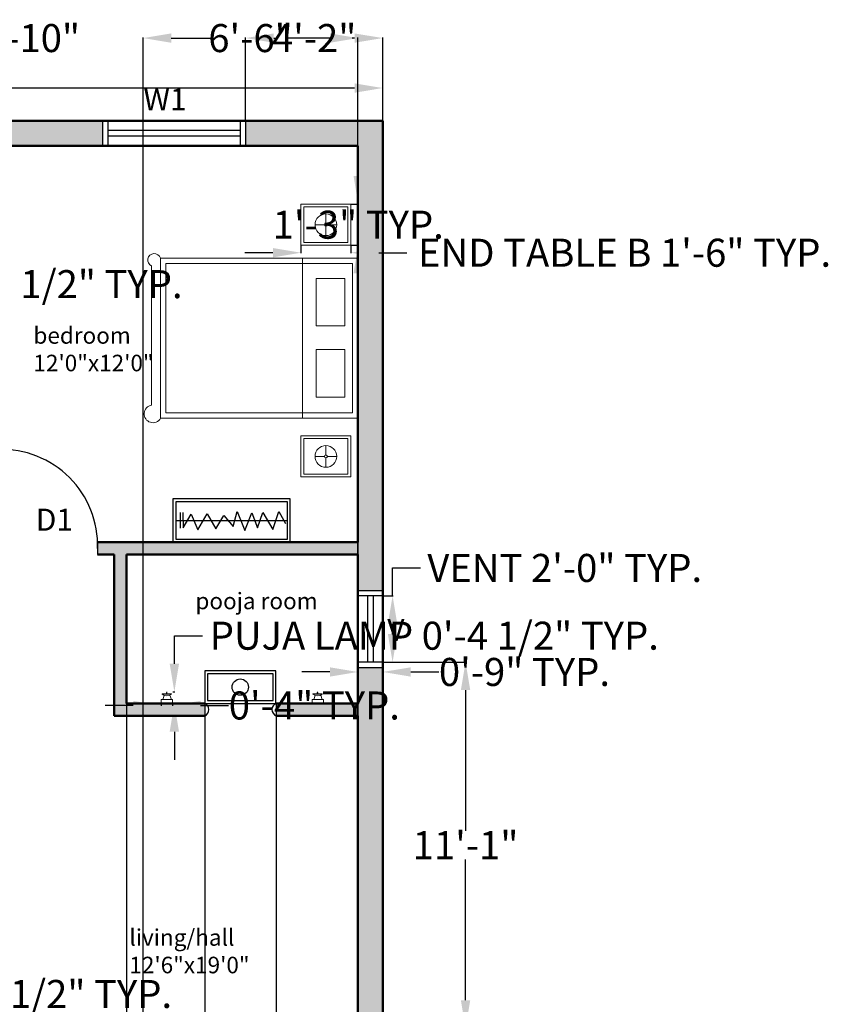
# Model space of a CAD drawing. Units: inches. Extents: x 2391 to 2964, y 130 to 798.
# Tile 4 of 4: x 2671 to 2964, y 431 to 789. Entities that reach past the tile are written whole.
import ezdxf

# ---------------------------------------------------------------- set-up
doc = ezdxf.new("R2010")
doc.units = ezdxf.units.IN
doc.header["$MEASUREMENT"] = 0
for name, color, linetype, lineweight in [('A-ANNO-DIMS', 2, 'Continuous', 18), ('A-ANNO-TEXT', 7, 'Continuous', 18), ('A-AREA-IDEN', 7, 'Continuous', 25), ('A-DOOR', 3, 'Continuous', 25), ('A-FLOR-CASE', 8, 'Continuous', 25), ('A-FURN', 8, 'Continuous', 18), ('A-GLAZ', 4, 'Continuous', 25), ('A-WALL', 7, 'Continuous', 50)]:
    doc.layers.add(name, color=color, linetype=linetype, lineweight=lineweight)
doc.layers.add('A-WALL-PATT', color=11, linetype='Continuous', lineweight=13, true_color=0xf27172)
doc.styles.get("Standard").update_dxf_attribs({"font": 'arial.ttf'})
doc.dimstyles.get("Standard").update_dxf_attribs({"dimtxt": 10.18, "dimasz": 10.18, "dimexe": 0.18, "dimexo": 0.0625, "dimgap": 0.09, "dimtad": 0, "dimtih": 1, "dimtoh": 1, "dimdec": 0, "dimzin": 0, "dimdsep": 46, "dimlunit": 3, "dimtxsty": 'Standard', "dimcen": 0.09, "dimadec": 0, "dimazin": 0, "dimtfac": 1, "dimtdec": 0, "dimtofl": 0, "dimtmove": 0, "dimatfit": 3, "dimfxl": 1, "dimtolj": 1, "dimtzin": 0, "dimarcsym": 0})

# ---------------------------------------------------------------- blocks, each defined once
blk = doc.blocks.new('*D3')
at = {"layer": 'A-ANNO-DIMS', "color": 0, "lineweight": -2, "transparency": 16777216}
for p, q in [((2502.4, 752.3), (2502.4, 764.38)), ((2512.58, 764.2), (2643.58, 764.2)), ((2792.22, 764.2), (2661.21, 764.2)), ((2802.4, 752.3), (2802.4, 764.38))]:
    blk.add_line(p, q, dxfattribs=at)
at = {"layer": 'A-ANNO-DIMS', "color": 0, "transparency": 16777216}
for points in [[(2512.58, 765.89), (2512.58, 762.5), (2502.4, 764.2)], [(2792.22, 765.89), (2792.22, 762.5), (2802.4, 764.2)]]:
    blk.add_solid(points, dxfattribs=at)
at = {"layer": 'Defpoints', "color": 0, "transparency": 16777216}
for p in [(2802.4, 764.2), (2502.4, 752.24), (2802.4, 752.24)]:
    blk.add_point(p, dxfattribs=at)
at = {"layer": 'A-ANNO-DIMS', "color": 0, "transparency": 16777216, "insert": (2652.4, 764.2), "char_height": 10.18, "attachment_point": 5}
blk.add_mtext("\\A1;25'", dxfattribs=at)
blk = doc.blocks.new('WIN-W1-48')
for p, q in [((0, 0), (0, 9)), ((2, 0), (2, 9)), ((50, 0), (50, 9)), ((52, 0), (52, 9)), ((2, 5.5), (50, 5.5)), ((2, 3.5), (50, 3.5))]:
    blk.add_line(p, q)
blk = doc.blocks.new('VENT-24')
for p, q in [((9, 24), (0, 24)), ((3.5, 24), (3.5, 0)), ((5.5, 24), (5.5, 0)), ((9, 0), (0, 0))]:
    blk.add_line(p, q)
blk = doc.blocks.new('DOOR-SWING-36')
for p, q in [((0, 4.5), (0, 38.25)), ((2, 2.25), (2, 38.25)), ((36, 4.5), (36, 0)), ((0, 2.25), (0, 0)), ((2, 2.25), (0, 2.25))]:
    blk.add_line(p, q)
blk.add_arc((1, 3.25), 35.01, 358.3634, 91.6366)
blk = doc.blocks.new('NIGHTSTAND-B')
for p, q in [((8.49, 7.46), (5.08, 7.46)), ((9.58, 7.46), (12.99, 7.46)), ((9.04, 6.92), (9.04, 3.51))]:
    blk.add_line(p, q)
for points in [[(0, 14.92), (18.07, 14.92), (18.07, 0), (0, 0)], [(1, 13.92), (17.07, 13.92), (17.07, 1), (1, 1)]]:
    blk.add_lwpolyline(points, close=True)
blk.add_lwpolyline([(9.04, 8.01), (9.04, 11.41)])
for radius in [3.95, 0.546]:
    blk.add_circle((9.04, 7.46), radius)
blk = doc.blocks.new('PUJA-LAMP')
for p, q in [((0, 1.56), (4.1, 1.54)), ((0, 1.56), (0, 0)), ((0.3, 3.46), (0.3, 3.53)), ((0.3, 3.53), (3.65, 3.52)), ((0.3, 3.46), (3.68, 3.45)), ((0.57, 1.56), (1.05, 3.01)), ((1.19, 3.45), (1.19, 3.46)), ((3.03, 3.45), (3.03, 3.46)), ((3.7, 1.56), (3.16, 3.11)), ((3.65, 3.52), (3.68, 3.52)), ((3.68, 3.52), (3.68, 3.52)), ((3.68, 3.52), (3.68, 3.45)), ((4.1, 1.54), (4.1, 0.12))]:
    blk.add_line(p, q)
for centre, radius, start, end in [((2.79, 3.92), 0.907, 153.661, 206.0678), ((1.19, 3.93), 0.884, 333.0647, 26.9353), ((1.99, 5.45), 2.62, 229.7155, 310.0133)]:
    blk.add_arc(centre, radius, start, end)
blk = doc.blocks.new('*D19')
at = {"layer": 'A-ANNO-DIMS', "color": 0, "lineweight": -2, "transparency": 16777216}
for p, q in [((2806, 579.74), (2806, 589.92)), ((2806, 589.92), (2816.18, 589.92)), ((2802.46, 579.74), (2806.18, 579.74)), ((2806, 565.92), (2806, 569.56)), ((2802.46, 555.74), (2806.18, 555.74))]:
    blk.add_line(p, q, dxfattribs=at)
at = {"layer": 'A-ANNO-DIMS', "color": 0, "transparency": 16777216}
for points in [[(2804.3, 569.56), (2807.7, 569.56), (2806, 579.74)], [(2804.3, 565.92), (2807.7, 565.92), (2806, 555.74)]]:
    blk.add_solid(points, dxfattribs=at)
at = {"layer": 'Defpoints', "color": 0, "transparency": 16777216}
for p in [(2802.4, 579.74), (2806, 579.74), (2802.4, 555.74)]:
    blk.add_point(p, dxfattribs=at)
at = {"layer": 'A-ANNO-DIMS', "color": 0, "transparency": 16777216, "insert": (2868.5, 589.92), "char_height": 10.18, "attachment_point": 5}
blk.add_mtext('\\A1;VENT 2\'-0" TYP.', dxfattribs=at)
blk = doc.blocks.new('*D20')
at = {"layer": 'A-ANNO-DIMS', "color": 0, "lineweight": -2, "transparency": 16777216}
for p, q in [((2793.4, 555.67), (2793.4, 551.96)), ((2802.4, 555.67), (2802.4, 551.96)), ((2783.22, 552.14), (2773.04, 552.14)), ((2812.58, 552.14), (2822.76, 552.14))]:
    blk.add_line(p, q, dxfattribs=at)
at = {"layer": 'A-ANNO-DIMS', "color": 0, "transparency": 16777216}
for points in [[(2783.22, 553.83), (2783.22, 550.44), (2793.4, 552.14)], [(2812.58, 553.83), (2812.58, 550.44), (2802.4, 552.14)]]:
    blk.add_solid(points, dxfattribs=at)
at = {"layer": 'Defpoints', "color": 0, "transparency": 16777216}
for p in [(2793.4, 555.74), (2802.4, 555.74), (2802.4, 552.14)]:
    blk.add_point(p, dxfattribs=at)
at = {"layer": 'A-ANNO-DIMS', "color": 0, "transparency": 16777216, "insert": (2853.88, 552.14), "char_height": 10.18, "attachment_point": 5}
blk.add_mtext('\\A1;0\'-9" TYP.', dxfattribs=at)
blk = doc.blocks.new('*D21')
at = {"layer": 'A-ANNO-DIMS', "color": 0, "lineweight": -2, "transparency": 16777216}
for p, q in [((2513.58, 694.49), (2513.58, 692.8)), ((2524.04, 694.49), (2524.04, 692.8)), ((2503.4, 692.98), (2493.22, 692.98)), ((2534.22, 692.98), (2544.4, 692.98))]:
    blk.add_line(p, q, dxfattribs=at)
at = {"layer": 'A-ANNO-DIMS', "color": 0, "transparency": 16777216}
for points in [[(2503.4, 694.68), (2503.4, 691.28), (2513.58, 692.98)], [(2534.22, 694.68), (2534.22, 691.28), (2524.04, 692.98)]]:
    blk.add_solid(points, dxfattribs=at)
at = {"layer": 'Defpoints', "color": 0, "transparency": 16777216}
for p in [(2513.58, 694.55), (2524.04, 694.55), (2524.04, 692.98)]:
    blk.add_point(p, dxfattribs=at)
at = {"layer": 'A-ANNO-DIMS', "color": 0, "transparency": 16777216, "insert": (2639.27, 692.98), "char_height": 10.18, "attachment_point": 5}
blk.add_mtext('\\A1;END TABLE A 0\'-10 1/2" TYP.', dxfattribs=at)
blk = doc.blocks.new('*D23')
at = {"layer": 'A-ANNO-DIMS', "color": 0, "lineweight": -2, "transparency": 16777216}
for p, q in [((2772.74, 707.04), (2772.74, 704.21)), ((2790.81, 707.04), (2790.81, 704.21)), ((2762.56, 704.39), (2752.38, 704.39)), ((2800.99, 704.39), (2811.17, 704.39))]:
    blk.add_line(p, q, dxfattribs=at)
at = {"layer": 'A-ANNO-DIMS', "color": 0, "transparency": 16777216}
for points in [[(2762.56, 706.08), (2762.56, 702.69), (2772.74, 704.39)], [(2800.99, 706.08), (2800.99, 702.69), (2790.81, 704.39)]]:
    blk.add_solid(points, dxfattribs=at)
at = {"layer": 'Defpoints', "color": 0, "transparency": 16777216}
for p in [(2772.74, 707.1), (2790.81, 707.1), (2790.81, 704.39)]:
    blk.add_point(p, dxfattribs=at)
at = {"layer": 'A-ANNO-DIMS', "color": 0, "transparency": 16777216, "insert": (2890.23, 704.39), "char_height": 10.18, "attachment_point": 5}
blk.add_mtext('\\A1;END TABLE B 1\'-6" TYP.', dxfattribs=at)
blk = doc.blocks.new('*D24')
at = {"layer": 'A-ANNO-DIMS', "color": 0, "lineweight": -2, "transparency": 16777216}
for p, q in [((2793.53, 732.2), (2793.53, 742.38)), ((2790.88, 722.02), (2793.71, 722.02)), ((2790.88, 707.1), (2793.71, 707.1)), ((2793.53, 696.92), (2793.53, 686.74))]:
    blk.add_line(p, q, dxfattribs=at)
at = {"layer": 'A-ANNO-DIMS', "color": 0, "transparency": 16777216}
for points in [[(2791.83, 732.2), (2795.22, 732.2), (2793.53, 722.02)], [(2791.83, 696.92), (2795.22, 696.92), (2793.53, 707.1)]]:
    blk.add_solid(points, dxfattribs=at)
at = {"layer": 'Defpoints', "color": 0, "transparency": 16777216}
for p in [(2790.81, 722.02), (2793.53, 722.02), (2790.81, 707.1)]:
    blk.add_point(p, dxfattribs=at)
at = {"layer": 'A-ANNO-DIMS', "color": 0, "transparency": 16777216, "insert": (2793.53, 714.56), "char_height": 10.18, "attachment_point": 5}
blk.add_mtext('\\A1;1\'-3" TYP.', dxfattribs=at)
blk = doc.blocks.new('*D25')
at = {"layer": 'A-ANNO-DIMS', "color": 0, "lineweight": -2, "transparency": 16777216}
for p, q in [((2518.03, 436.55), (2518.03, 435.02)), ((2527.43, 436.55), (2527.43, 435.02)), ((2507.85, 435.2), (2497.67, 435.2)), ((2537.61, 435.2), (2547.79, 435.2))]:
    blk.add_line(p, q, dxfattribs=at)
at = {"layer": 'A-ANNO-DIMS', "color": 0, "transparency": 16777216}
for points in [[(2507.85, 436.9), (2507.85, 433.5), (2518.03, 435.2)], [(2537.61, 436.9), (2537.61, 433.5), (2527.43, 435.2)]]:
    blk.add_solid(points, dxfattribs=at)
at = {"layer": 'Defpoints', "color": 0, "transparency": 16777216}
for p in [(2518.03, 436.61), (2527.43, 436.61), (2527.43, 435.2)]:
    blk.add_point(p, dxfattribs=at)
at = {"layer": 'A-ANNO-DIMS', "color": 0, "transparency": 16777216, "insert": (2639.1, 435.2), "char_height": 10.18, "attachment_point": 5}
blk.add_mtext('\\A1;END TABLE C 0\'-9 1/2" TYP.', dxfattribs=at)
blk = doc.blocks.new('*D31')
at = {"layer": 'A-ANNO-DIMS', "color": 0, "lineweight": -2, "transparency": 16777216}
for p, q in [((2726.76, 555.13), (2726.76, 565.31)), ((2726.76, 565.31), (2736.94, 565.31)), ((2726.17, 544.95), (2726.94, 544.95)), ((2726.17, 540.62), (2726.94, 540.62)), ((2726.76, 530.44), (2726.76, 520.26))]:
    blk.add_line(p, q, dxfattribs=at)
at = {"layer": 'A-ANNO-DIMS', "color": 0, "transparency": 16777216}
for points in [[(2725.06, 555.13), (2728.46, 555.13), (2726.76, 544.95)], [(2725.06, 530.44), (2728.46, 530.44), (2726.76, 540.62)]]:
    blk.add_solid(points, dxfattribs=at)
at = {"layer": 'Defpoints', "color": 0, "transparency": 16777216}
for p in [(2726.11, 544.95), (2726.76, 544.95), (2726.11, 540.62)]:
    blk.add_point(p, dxfattribs=at)
at = {"layer": 'A-ANNO-DIMS', "color": 0, "transparency": 16777216, "insert": (2821.15, 565.31), "char_height": 10.18, "attachment_point": 5}
blk.add_mtext('\\A1;PUJA LAMP 0\'-4 1/2" TYP.', dxfattribs=at)
blk = doc.blocks.new('*D32')
at = {"layer": 'A-ANNO-DIMS', "color": 0, "lineweight": -2, "transparency": 16777216}
for p, q in [((2711.84, 539.97), (2701.66, 539.97)), ((2722.02, 540.56), (2722.02, 539.79)), ((2726.11, 540.56), (2726.11, 539.79)), ((2736.29, 539.97), (2746.47, 539.97))]:
    blk.add_line(p, q, dxfattribs=at)
at = {"layer": 'A-ANNO-DIMS', "color": 0, "transparency": 16777216}
for points in [[(2711.84, 541.67), (2711.84, 538.27), (2722.02, 539.97)], [(2736.29, 541.67), (2736.29, 538.27), (2726.11, 539.97)]]:
    blk.add_solid(points, dxfattribs=at)
at = {"layer": 'Defpoints', "color": 0, "transparency": 16777216}
for p in [(2722.02, 540.62), (2726.11, 540.62), (2726.11, 539.97)]:
    blk.add_point(p, dxfattribs=at)
at = {"layer": 'A-ANNO-DIMS', "color": 0, "transparency": 16777216, "insert": (2777.59, 539.97), "char_height": 10.18, "attachment_point": 5}
blk.add_mtext('\\A1;0\'-4" TYP.', dxfattribs=at)
blk = doc.blocks.new('*D33')
at = {"layer": 'A-ANNO-DIMS', "color": 0, "lineweight": -2, "transparency": 16777216}
for p, q in [((2659.9, 743.17), (2659.9, 145.07)), ((2793.4, 743.17), (2793.4, 145.07)), ((2670.08, 145.25), (2697.69, 145.25)), ((2783.22, 145.25), (2755.61, 145.25))]:
    blk.add_line(p, q, dxfattribs=at)
at = {"layer": 'A-ANNO-DIMS', "color": 0, "transparency": 16777216}
for points in [[(2670.08, 146.95), (2670.08, 143.56), (2659.9, 145.25)], [(2783.22, 146.95), (2783.22, 143.56), (2793.4, 145.25)]]:
    blk.add_solid(points, dxfattribs=at)
at = {"layer": 'Defpoints', "color": 0, "transparency": 16777216}
for p in [(2659.9, 743.24), (2793.4, 743.24), (2793.4, 145.25)]:
    blk.add_point(p, dxfattribs=at)
at = {"layer": 'A-ANNO-DIMS', "color": 0, "transparency": 16777216, "insert": (2726.65, 145.25), "char_height": 10.18, "attachment_point": 5}
blk.add_mtext('\\A1;11\'-1 1/2"', dxfattribs=at)
blk = doc.blocks.new('*D36')
at = {"layer": 'A-ANNO-DIMS', "color": 0, "lineweight": -2, "transparency": 16777216}
for p, q in [((2709.4, 594.67), (2709.4, 145.07)), ((2793.4, 594.67), (2793.4, 145.07)), ((2719.58, 145.25), (2737.82, 145.25)), ((2783.22, 145.25), (2764.98, 145.25))]:
    blk.add_line(p, q, dxfattribs=at)
at = {"layer": 'A-ANNO-DIMS', "color": 0, "transparency": 16777216}
for points in [[(2719.58, 146.95), (2719.58, 143.56), (2709.4, 145.25)], [(2783.22, 146.95), (2783.22, 143.56), (2793.4, 145.25)]]:
    blk.add_solid(points, dxfattribs=at)
at = {"layer": 'Defpoints', "color": 0, "transparency": 16777216}
for p in [(2709.4, 594.74), (2793.4, 594.74), (2793.4, 145.25)]:
    blk.add_point(p, dxfattribs=at)
at = {"layer": 'A-ANNO-DIMS', "color": 0, "transparency": 16777216, "insert": (2751.4, 145.25), "char_height": 10.18, "attachment_point": 5}
blk.add_mtext('\\A1;7\'-0"', dxfattribs=at)
blk = doc.blocks.new('*D38')
at = {"layer": 'A-ANNO-DIMS', "color": 0, "lineweight": -2, "transparency": 16777216}
for p, q in [((2752.65, 752.3), (2752.65, 782.52)), ((2762.83, 782.34), (2763.7, 782.34)), ((2792.22, 782.34), (2791.35, 782.34)), ((2802.4, 752.3), (2802.4, 782.52))]:
    blk.add_line(p, q, dxfattribs=at)
at = {"layer": 'A-ANNO-DIMS', "color": 0, "transparency": 16777216}
for points in [[(2762.83, 784.03), (2762.83, 780.64), (2752.65, 782.34)], [(2792.22, 784.03), (2792.22, 780.64), (2802.4, 782.34)]]:
    blk.add_solid(points, dxfattribs=at)
at = {"layer": 'Defpoints', "color": 0, "transparency": 16777216}
for p in [(2802.4, 782.34), (2752.65, 752.24), (2802.4, 752.24)]:
    blk.add_point(p, dxfattribs=at)
at = {"layer": 'A-ANNO-DIMS', "color": 0, "transparency": 16777216, "insert": (2777.52, 782.34), "char_height": 10.18, "attachment_point": 5}
blk.add_mtext('\\A1;4\'-2"', dxfattribs=at)
blk = doc.blocks.new('*D43')
at = {"layer": 'A-ANNO-DIMS', "color": 0, "lineweight": -2, "transparency": 16777216}
for p, q in [((2802.46, 555.74), (2832.68, 555.74)), ((2832.5, 545.56), (2832.5, 494.44)), ((2832.5, 432.92), (2832.5, 484.03)), ((2802.46, 422.74), (2832.68, 422.74))]:
    blk.add_line(p, q, dxfattribs=at)
at = {"layer": 'A-ANNO-DIMS', "color": 0, "transparency": 16777216}
for points in [[(2830.8, 545.56), (2834.2, 545.56), (2832.5, 555.74)], [(2830.8, 432.92), (2834.2, 432.92), (2832.5, 422.74)]]:
    blk.add_solid(points, dxfattribs=at)
at = {"layer": 'Defpoints', "color": 0, "transparency": 16777216}
for p in [(2802.4, 555.74), (2832.5, 555.74), (2802.4, 422.74)]:
    blk.add_point(p, dxfattribs=at)
at = {"layer": 'A-ANNO-DIMS', "color": 0, "transparency": 16777216, "insert": (2832.5, 489.24), "char_height": 10.18, "attachment_point": 5}
blk.add_mtext('\\A1;11\'-1"', dxfattribs=at)
blk = doc.blocks.new('*D44')
at = {"layer": 'A-ANNO-DIMS', "color": 0, "lineweight": -2, "transparency": 16777216}
for p, q in [((2715.45, 257.3), (2715.45, 782.52)), ((2725.63, 782.34), (2740.78, 782.34)), ((2783.22, 782.34), (2768.07, 782.34)), ((2793.4, 257.3), (2793.4, 782.52))]:
    blk.add_line(p, q, dxfattribs=at)
at = {"layer": 'A-ANNO-DIMS', "color": 0, "transparency": 16777216}
for points in [[(2725.63, 784.03), (2725.63, 780.64), (2715.45, 782.34)], [(2783.22, 784.03), (2783.22, 780.64), (2793.4, 782.34)]]:
    blk.add_solid(points, dxfattribs=at)
at = {"layer": 'Defpoints', "color": 0, "transparency": 16777216}
for p in [(2793.4, 782.34), (2715.45, 257.24), (2793.4, 257.24)]:
    blk.add_point(p, dxfattribs=at)
at = {"layer": 'A-ANNO-DIMS', "color": 0, "transparency": 16777216, "insert": (2754.42, 782.34), "char_height": 10.18, "attachment_point": 5}
blk.add_mtext('\\A1;6\'-6"', dxfattribs=at)
blk = doc.blocks.new('*D46')
at = {"layer": 'A-ANNO-DIMS', "color": 0, "lineweight": -2, "transparency": 16777216}
for p, q in [((2737.79, 536.17), (2737.79, 145.07)), ((2763.73, 536.17), (2763.73, 145.07)), ((2747.97, 145.25), (2753.55, 145.25)), ((2763.73, 145.25), (2773.91, 145.25))]:
    blk.add_line(p, q, dxfattribs=at)
at = {"layer": 'A-ANNO-DIMS', "color": 0, "transparency": 16777216}
for points in [[(2747.97, 146.95), (2747.97, 143.56), (2737.79, 145.25)], [(2753.55, 146.95), (2753.55, 143.56), (2763.73, 145.25)]]:
    blk.add_solid(points, dxfattribs=at)
at = {"layer": 'Defpoints', "color": 0, "transparency": 16777216}
for p in [(2737.79, 536.24), (2763.73, 536.24), (2763.73, 145.25)]:
    blk.add_point(p, dxfattribs=at)
at = {"layer": 'A-ANNO-DIMS', "color": 0, "transparency": 16777216, "insert": (2787.61, 145.25), "char_height": 10.18, "attachment_point": 5}
blk.add_mtext('\\A1;2\'-2"', dxfattribs=at)
blk = doc.blocks.new('*D52')
at = {"layer": 'A-ANNO-DIMS', "color": 0, "lineweight": -2, "transparency": 16777216}
for p, q in [((2615.22, 782.34), (2605.04, 782.34)), ((2625.4, 311.3), (2625.4, 782.52)), ((2635.4, 311.3), (2635.4, 782.52)), ((2645.58, 782.34), (2655.76, 782.34))]:
    blk.add_line(p, q, dxfattribs=at)
at = {"layer": 'A-ANNO-DIMS', "color": 0, "transparency": 16777216}
for points in [[(2615.22, 784.03), (2615.22, 780.64), (2625.4, 782.34)], [(2645.58, 784.03), (2645.58, 780.64), (2635.4, 782.34)]]:
    blk.add_solid(points, dxfattribs=at)
at = {"layer": 'Defpoints', "color": 0, "transparency": 16777216}
for p in [(2635.4, 782.34), (2625.4, 311.24), (2635.4, 311.24)]:
    blk.add_point(p, dxfattribs=at)
at = {"layer": 'A-ANNO-DIMS', "color": 0, "transparency": 16777216, "insert": (2673.33, 782.34), "char_height": 10.18, "attachment_point": 5}
blk.add_mtext('\\A1;0\'-10"', dxfattribs=at)

msp = doc.modelspace()

# ---------------------------------------------------------------- hatches: boundary and pattern name
at = {"layer": 'A-WALL-PATT'}
h = msp.add_hatch(color=256, dxfattribs=at)
h.dxf.hatch_style = 1
h.paths.add_polyline_path([(2557.4, 752.24), (2502.4, 752.24), (2502.4, 579.74), (2511.4, 579.74), (2511.4, 594.74), (2595.4, 594.74), (2599.9, 594.74), (2616.4, 594.74), (2616.4, 596.99, -0.014283), (2616.4, 598.99), (2616.4, 599.24), (2511.4, 599.24), (2511.4, 743.24), (2557.4, 743.24)])
h.paths.add_polyline_path([(2700.65, 752.24), (2609.4, 752.24), (2609.4, 743.24), (2655.4, 743.24), (2655.4, 599.24), (2650.4, 599.24), (2650.4, 596.99), (2652.4, 596.99), (2652.4, 594.74), (2662.9, 594.74), (2662.9, 596.99), (2664.9, 596.99), (2664.9, 599.24), (2659.9, 599.24), (2659.9, 743.24), (2700.65, 743.24)])
h.paths.add_polyline_path([(2802.4, 752.24), (2752.65, 752.24), (2752.65, 743.24), (2793.4, 743.24), (2793.4, 599.24), (2698.9, 599.24), (2698.9, 598.99, -0.014283), (2698.9, 596.99), (2698.9, 594.74), (2704.9, 594.74), (2704.9, 536.24), (2737.79, 536.24), (2737.79, 540.74), (2709.4, 540.74), (2709.4, 594.74), (2793.4, 594.74), (2793.4, 581.74), (2802.4, 581.74)])
h.paths.add_polyline_path([(2511.4, 444.24), (2502.4, 444.24), (2502.4, 383.74), (2511.4, 383.74), (2511.4, 399.74), (2655.4, 399.74), (2655.4, 354.74), (2655.65, 354.74, -0.014283), (2657.65, 354.74), (2659.9, 354.74), (2659.9, 407.24), (2657.65, 407.24), (2657.65, 409.24), (2655.4, 409.24), (2655.4, 404.24), (2511.4, 404.24)])
h.paths.add_polyline_path([(2511.4, 536.24), (2599.9, 536.24), (2655.4, 536.24), (2655.4, 443.24), (2655.65, 443.24, -0.014283), (2657.65, 443.24), (2659.9, 443.24), (2659.9, 540.74), (2599.9, 540.74), (2599.9, 555.74), (2597.65, 555.74, -0.014283), (2595.65, 555.74), (2595.4, 555.74), (2595.4, 540.74), (2511.4, 540.74), (2511.4, 555.74), (2502.4, 555.74), (2502.4, 496.24), (2511.4, 496.24), (2511.4, 503.82)])
h.paths.add_polyline_path([(2676.45, 257.24), (2511.4, 257.24), (2511.4, 311.24), (2659.9, 311.24), (2659.9, 318.74), (2657.65, 318.74), (2657.65, 320.74), (2655.4, 320.74), (2655.4, 315.74), (2511.4, 315.74), (2511.4, 331.74), (2502.4, 331.74), (2502.4, 248.24), (2676.45, 248.24)])
h.paths.add_polyline_path([(2802.4, 370.74), (2793.4, 370.74), (2793.4, 257.24), (2787.63, 257.24), (2787.63, 248.24), (2802.4, 248.24)])
h.paths.add_polyline_path([(2735.63, 257.24), (2715.45, 257.24), (2715.45, 254.74, -0.014283), (2715.45, 252.74), (2715.45, 248.24), (2721.55, 248.24), (2735.63, 248.24)])
h.paths.add_polyline_path([(2802.4, 553.74), (2793.4, 553.74), (2793.4, 540.74), (2763.73, 540.74), (2763.73, 536.24), (2793.4, 536.24), (2793.4, 422.74), (2802.4, 422.74)])

# ---------------------------------------------------------------- linework, layer by layer
at = {"layer": 'A-DOOR'}
for p, q in [((2737.79, 540.74), (2737.79, 536.24)), ((2763.73, 540.74), (2763.73, 536.24))]:
    msp.add_line(p, q, dxfattribs=at)
for centre, radius, start, end in [((2736.87, 538.49), 2.43, 292.2477, 67.7523), ((2764.62, 538.49), 2.42, 111.7537, 248.2463)]:
    msp.add_arc(centre, radius, start, end, dxfattribs=at)
at = {"layer": 'A-FLOR-CASE'}
for p, q in [((2728.87, 610.02), (2728.87, 604.41)), ((2729.83, 610.02), (2729.99, 604.44)), ((2729.99, 604.44), (2732.86, 609.41)), ((2732.86, 609.41), (2735.29, 603.72)), ((2735.29, 603.72), (2738.66, 609.55)), ((2738.66, 609.55), (2741.82, 604.07)), ((2741.82, 604.07), (2744.67, 609)), ((2744.67, 609), (2748.12, 605.01)), ((2748.12, 605.01), (2749.58, 610.36)), ((2749.58, 610.36), (2752.38, 603.51)), ((2752.38, 603.51), (2754.93, 609.94)), ((2754.93, 609.94), (2757.01, 604.5)), ((2757.01, 604.5), (2758.88, 610.05)), ((2758.88, 610.05), (2762.47, 603.83)), ((2762.47, 603.83), (2764.65, 610.41)), ((2764.65, 610.41), (2767.15, 606.08)), ((2727.37, 607.16), (2767.7, 607.16))]:
    msp.add_line(p, q, dxfattribs=at)
for points in [[(2768.7, 599.24), (2726.37, 599.24), (2726.37, 615.09), (2768.7, 615.09)], [(2767.7, 600.24), (2727.37, 600.24), (2727.37, 614.09), (2767.7, 614.09)], [(2737.79, 540.74), (2763.59, 540.74), (2763.59, 552.52), (2737.79, 552.52)], [(2738.79, 541.74), (2762.59, 541.74), (2762.59, 551.52), (2738.79, 551.52)]]:
    msp.add_lwpolyline(points, close=True, dxfattribs=at)
msp.add_circle((2750.69, 546.63), 2.96, dxfattribs=at)
at = {"layer": 'A-FURN'}
for p, q in [((2773.3, 702.44), (2773.3, 644.26)), ((2718.5, 699.61), (2718.5, 649.02))]:
    msp.add_line(p, q, dxfattribs=at)
for points in [[(2793.4, 702.44), (2721.69, 702.44), (2721.69, 644.26), (2793.4, 644.26)], [(2791.4, 700.44), (2723.69, 700.44), (2723.69, 646.26), (2791.4, 646.26)], [(2778.21, 695.08), (2788.69, 695.08), (2788.69, 677.81), (2778.21, 677.81)], [(2778.21, 669.26), (2788.69, 669.26), (2788.69, 651.99), (2778.21, 651.99)]]:
    msp.add_lwpolyline(points, close=True, dxfattribs=at)
for centre, radius, start, end in [((2719.45, 701.75), 2.34, 17.1817, 245.9572), ((2718.99, 645.86), 3.2, 98.8565, 330.0452)]:
    msp.add_arc(centre, radius, start, end, dxfattribs=at)
at = {"layer": 'A-GLAZ'}
for p, q in [((2793.4, 581.74), (2802.4, 581.74)), ((2793.4, 553.74), (2802.4, 553.74))]:
    msp.add_line(p, q, dxfattribs=at)
at = {"layer": 'A-WALL'}
for p, q in [((2502.4, 752.24), (2802.4, 752.24)), ((2802.4, 752.24), (2802.4, 248.24)), ((2659.9, 743.24), (2793.4, 743.24)), ((2793.4, 743.24), (2793.4, 599.24)), ((2698.89, 599.24), (2793.4, 599.24)), ((2698.9, 594.74), (2704.9, 594.74)), ((2704.9, 594.74), (2704.9, 536.24)), ((2709.4, 594.74), (2709.4, 540.74)), ((2709.4, 594.74), (2793.4, 594.74)), ((2793.4, 594.74), (2793.4, 540.74)), ((2709.4, 540.74), (2737.79, 540.74)), ((2763.73, 540.74), (2793.4, 540.74)), ((2704.9, 536.24), (2737.79, 536.24)), ((2763.73, 536.24), (2793.4, 536.24)), ((2793.4, 536.24), (2793.4, 257.24))]:
    msp.add_line(p, q, dxfattribs=at)

# ---------------------------------------------------------------- block references
at = {"layer": 'A-DOOR'}
msp.add_blockref('DOOR-SWING-36', (2662.9, 594.74), dxfattribs=at)
at = {"layer": 'A-FURN'}
for name, p in [('NIGHTSTAND-B', (2772.74, 707.1)), ('NIGHTSTAND-B', (2772.74, 622.96)), ('PUJA-LAMP', (2722.01, 540.62)), ('PUJA-LAMP', (2776.79, 540.62))]:
    msp.add_blockref(name, p, dxfattribs=at)
at = {"layer": 'A-GLAZ', "rotation": 180}
msp.add_blockref('WIN-W1-48', (2752.65, 752.24), dxfattribs=at)
at = {"layer": 'A-GLAZ'}
msp.add_blockref('VENT-24', (2793.4, 555.74), dxfattribs=at)

# ---------------------------------------------------------------- texts
at = {"layer": 'A-ANNO-TEXT', "char_height": 8, "attachment_point": 1}
for s, insert in [('W1', (2715.55, 764.07)), ('D1', (2676.43, 611.44)), ('V', (2804.06, 571.42))]:
    msp.add_mtext_dynamic_manual_height_columns(s, width=35.9617, gutter_width=1, heights=[0], dxfattribs=dict(at, insert=insert))
at = {"layer": 'A-AREA-IDEN', "char_height": 6, "attachment_point": 1}
for s, insert in [('bedroom\\P12\'0"x12\'0"', (2675.59, 677.34)), ('pooja room', (2734.41, 580.92)), ('living/hall\\P12\'6"x19\'0"', (2710.43, 458.72))]:
    msp.add_mtext_dynamic_manual_height_columns(s, width=87.7895, gutter_width=1, heights=[0], dxfattribs=dict(at, insert=insert))

# ---------------------------------------------------------------- dimensions: what is measured, and where the dimension line sits
at = {"layer": 'A-ANNO-DIMS'}
for base, p1, p2, override, picture, middle in [((2635.4, 782.34), (2625.4, 311.24), (2635.4, 311.24), {"dimdec": 1, "dimlfac": 1, "dimrnd": 0, "dimzin": 1, "dimdsep": 46, "dimlunit": 4, "dimfrac": 2}, '*D52', (2673.33, 782.34)), ((2793.3997, 782.3351), (2715.4471, 257.2351), (2793.3997, 257.2351), {"dimdec": 1, "dimlfac": 1, "dimrnd": 0, "dimzin": 1, "dimdsep": 46, "dimlunit": 4, "dimfrac": 2}, '*D44', (2754.4234, 782.3351)), ((2802.399651, 782.335057), (2752.649651, 752.235057), (2802.399651, 752.235057), {"dimdec": 1, "dimlfac": 1, "dimrnd": 0, "dimzin": 1, "dimdsep": 46, "dimlunit": 4, "dimfrac": 2}, '*D38', (2777.524651, 782.335057)), ((2802.4, 764.2), (2502.4, 752.24), (2802.4, 752.24), {"dimclrd": 0, "dimclre": 0, "dimclrt": 0}, '*D3', (2652.4, 764.2)), ((2793.4, 145.25), (2659.9, 743.24), (2793.4, 743.24), {"dimdec": 1, "dimlfac": 1, "dimrnd": 0, "dimzin": 1, "dimdsep": 46, "dimlunit": 4, "dimfrac": 2}, '*D33', (2726.65, 145.25)), ((2793.4, 145.25), (2709.4, 594.74), (2793.4, 594.74), {"dimdec": 1, "dimlfac": 1, "dimrnd": 0, "dimzin": 1, "dimdsep": 46, "dimlunit": 4, "dimfrac": 2}, '*D36', (2751.4, 145.25)), ((2763.73, 145.25), (2737.79, 536.24), (2763.73, 536.24), {"dimdec": 1, "dimlfac": 1, "dimrnd": 0, "dimzin": 1, "dimdsep": 46, "dimlunit": 4, "dimfrac": 2}, '*D46', (2787.61, 145.25))]:
    dim = msp.add_linear_dim(base=base, p1=p1, p2=p2, dimstyle='Standard', override=override, dxfattribs=at)
    dim.commit()
    dim.dimension.update_dxf_attribs({"geometry": picture, "text_midpoint": middle})
for base, p1, p2, text, picture, middle in [((2790.81, 704.39), (2772.74, 707.1), (2790.81, 707.1), 'END TABLE B <> TYP.', '*D23', (2890.23, 704.39)), ((2524.04, 692.98), (2513.58, 694.55), (2524.04, 694.55), 'END TABLE A <> TYP.', '*D21', (2639.27, 692.98)), ((2802.4, 552.14), (2793.4, 555.74), (2802.4, 555.74), '<> TYP.', '*D20', (2853.88, 552.14)), ((2726.11, 539.97), (2722.02, 540.62), (2726.11, 540.62), '<> TYP.', '*D32', (2777.59, 539.97)), ((2527.43, 435.2), (2518.03, 436.61), (2527.43, 436.61), 'END TABLE C <> TYP.', '*D25', (2639.1, 435.2))]:
    dim = msp.add_linear_dim(base=base, p1=p1, p2=p2, text=text, dimstyle='Standard', override={"dimdec": 1, "dimlfac": 1, "dimrnd": 0, "dimzin": 1, "dimdsep": 46, "dimlunit": 4, "dimfrac": 2}, dxfattribs=at)
    dim.commit()
    dim.dimension.update_dxf_attribs({"geometry": picture, "text_midpoint": middle})
for base, p1, p2, text, picture, middle in [((2793.53, 722.02), (2790.81, 707.1), (2790.81, 722.02), '<> TYP.', '*D24', (2793.53, 714.56)), ((2806, 579.74), (2802.4, 555.74), (2802.4, 579.74), 'VENT <> TYP.', '*D19', (2868.5, 589.92)), ((2726.76, 544.95), (2726.11, 540.62), (2726.11, 544.95), 'PUJA LAMP <> TYP.', '*D31', (2821.15, 565.31))]:
    dim = msp.add_linear_dim(base=base, p1=p1, p2=p2, angle=90, text=text, dimstyle='Standard', override={"dimdec": 1, "dimlfac": 1, "dimrnd": 0, "dimzin": 1, "dimdsep": 46, "dimlunit": 4, "dimfrac": 2}, dxfattribs=at)
    dim.commit()
    dim.dimension.update_dxf_attribs({"geometry": picture, "text_midpoint": middle})
dim = msp.add_linear_dim(base=(2832.5, 555.74), p1=(2802.4, 422.74), p2=(2802.4, 555.74), angle=90, dimstyle='Standard', override={"dimdec": 1, "dimlfac": 1, "dimrnd": 0, "dimzin": 1, "dimdsep": 46, "dimlunit": 4, "dimfrac": 2}, dxfattribs=at)
dim.commit()
dim.dimension.update_dxf_attribs({"geometry": '*D43', "text_midpoint": (2832.5, 489.24)})

doc.saveas('drawing.dxf')
